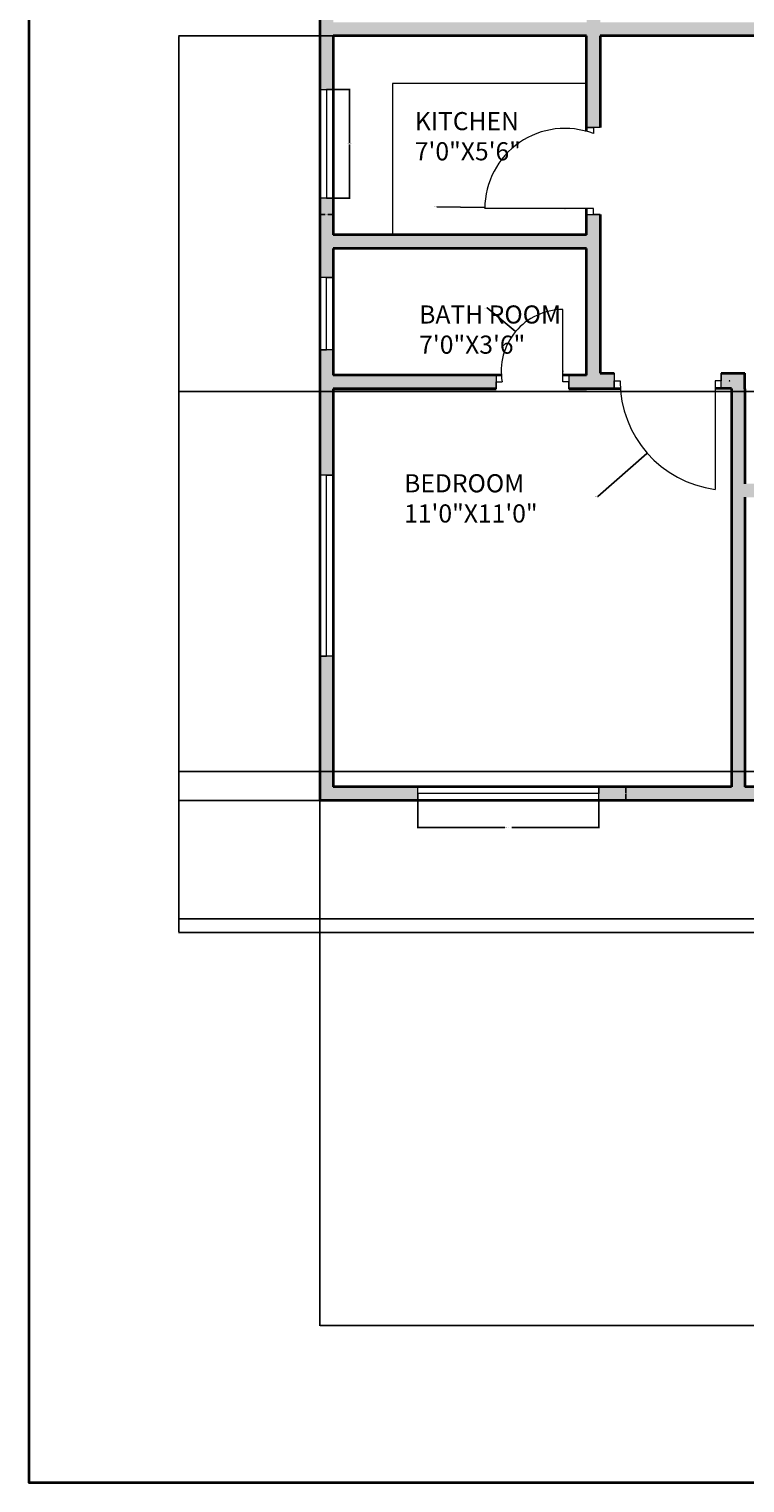
# Model space of a CAD drawing. Units: inches. Extents: x 2314 to 3223, y 1382 to 2735.
# Tile 1 of 14: x 2314 to 2551, y 1382 to 1864. Entities that reach past the tile are written whole.
import ezdxf

# ---------------------------------------------------------------- set-up
doc = ezdxf.new("R2010")
doc.units = ezdxf.units.IN
for name, color, linetype, lineweight in [('A-ANNO-DIMS', 2, 'Continuous', 18), ('A-ANNO-TTLB', 7, 'Continuous', 35), ('A-AREA-IDEN', 7, 'Continuous', 18), ('A-DOOR', 3, 'Continuous', 18), ('A-FLOR-FIXT', 8, 'Continuous', 18), ('A-GLAZ', 4, 'Continuous', 18), ('A-WALL', 7, 'Continuous', 35)]:
    doc.layers.add(name, color=color, linetype=linetype, lineweight=lineweight)
doc.layers.add('A-WALL-PATT', color=251, linetype='Continuous', lineweight=13, true_color=0x636466)
doc.styles.get("Standard").update_dxf_attribs({"font": 'arial.ttf'})
doc.dimstyles.get("Standard").update_dxf_attribs({"dimtxt": 0.18, "dimasz": 0.18, "dimexe": 0.18, "dimexo": 0.0625, "dimgap": 0.09, "dimtad": 0, "dimtih": 1, "dimtoh": 1, "dimdec": 4, "dimzin": 0, "dimdsep": 46, "dimtxsty": 'Standard', "dimcen": 0.09, "dimadec": 0, "dimazin": 0, "dimtfac": 1, "dimtdec": 4, "dimtofl": 0, "dimtmove": 0, "dimatfit": 3, "dimfxl": 1, "dimtolj": 1, "dimtzin": 0, "dimarcsym": 0})

# ---------------------------------------------------------------- blocks, each defined once
blk = doc.blocks.new('WIN-PLAN-24')
for p, q in [((0, 24), (4.5, 24)), ((4.5, 24), (2.25, 24)), ((2.25, 24), (2.25, 0)), ((2.25, 0), (0, 0)), ((0, 0), (4.5, 0))]:
    blk.add_line(p, q)
blk = doc.blocks.new('WIN-PLAN-60')
for p, q in [((0, 4.5), (0, 0)), ((0, 0), (0, 2.25)), ((0, 2.25), (60, 2.25)), ((60, 2.25), (60, 4.5)), ((60, 4.5), (60, 0))]:
    blk.add_line(p, q)
blk = doc.blocks.new('WIN-PLAN-36-ALT')
for p, q in [((0, 36), (4.5, 36)), ((4.5, 36), (2.25, 36)), ((2.25, 36), (2.25, 0)), ((4.5, 0), (0, 0)), ((2.25, 0), (4.5, 0))]:
    blk.add_line(p, q)
blk = doc.blocks.new('*D11')
at = {"layer": 'A-ANNO-DIMS', "color": 0, "lineweight": -2, "transparency": 16777216}
for p, q in [((2442.93, 1608.32), (2442.93, 1599.2)), ((2502.93, 1608.32), (2502.93, 1599.2)), ((2443.11, 1599.38), (2471.82, 1599.38)), ((2502.75, 1599.38), (2474.05, 1599.38))]:
    blk.add_line(p, q, dxfattribs=at)
at = {"layer": 'A-ANNO-DIMS', "color": 0, "transparency": 16777216}
for points in [[(2443.11, 1599.41), (2443.11, 1599.35), (2442.93, 1599.38)], [(2502.75, 1599.41), (2502.75, 1599.35), (2502.93, 1599.38)]]:
    blk.add_solid(points, dxfattribs=at)
at = {"layer": 'Defpoints', "color": 0, "transparency": 16777216}
for p in [(2442.93, 1608.38), (2502.93, 1608.38), (2442.93, 1599.38)]:
    blk.add_point(p, dxfattribs=at)
at = {"layer": 'A-ANNO-DIMS', "color": 0, "transparency": 16777216, "insert": (2472.93, 1599.38), "char_height": 0.18, "attachment_point": 5}
blk.add_mtext('\\A1;WINDOW 60 TYP.', dxfattribs=at)
blk = doc.blocks.new('*D12')
at = {"layer": 'A-ANNO-DIMS', "color": 0, "lineweight": -2, "transparency": 16777216}
for p, q in [((2503, 1612.88), (2512.11, 1612.88)), ((2511.93, 1612.7), (2511.93, 1610.81)), ((2511.93, 1608.56), (2511.93, 1610.45)), ((2503, 1608.38), (2512.11, 1608.38))]:
    blk.add_line(p, q, dxfattribs=at)
at = {"layer": 'A-ANNO-DIMS', "color": 0, "transparency": 16777216}
for points in [[(2511.9, 1612.7), (2511.96, 1612.7), (2511.93, 1612.88)], [(2511.9, 1608.56), (2511.96, 1608.56), (2511.93, 1608.38)]]:
    blk.add_solid(points, dxfattribs=at)
at = {"layer": 'Defpoints', "color": 0, "transparency": 16777216}
for p in [(2502.93, 1612.88), (2502.93, 1608.38), (2511.93, 1608.38)]:
    blk.add_point(p, dxfattribs=at)
at = {"layer": 'A-ANNO-DIMS', "color": 0, "transparency": 16777216, "insert": (2511.93, 1610.63), "char_height": 0.18, "attachment_point": 5}
blk.add_mtext('\\A1;5 TYP.', dxfattribs=at)
blk = doc.blocks.new('*D19')
at = {"layer": 'A-ANNO-DIMS', "color": 0, "lineweight": -2, "transparency": 16777216}
for p, q in [((2414.96, 1844.09), (2420.47, 1844.09)), ((2420.29, 1843.91), (2420.29, 1826.28)), ((2420.29, 1808.27), (2420.29, 1825.91)), ((2414.96, 1808.09), (2420.47, 1808.09))]:
    blk.add_line(p, q, dxfattribs=at)
at = {"layer": 'A-ANNO-DIMS', "color": 0, "transparency": 16777216}
for points in [[(2420.26, 1843.91), (2420.32, 1843.91), (2420.29, 1844.09)], [(2420.26, 1808.27), (2420.32, 1808.27), (2420.29, 1808.09)]]:
    blk.add_solid(points, dxfattribs=at)
at = {"layer": 'Defpoints', "color": 0, "transparency": 16777216}
for p in [(2414.89, 1844.09), (2420.29, 1844.09), (2414.89, 1808.09)]:
    blk.add_point(p, dxfattribs=at)
at = {"layer": 'A-ANNO-DIMS', "color": 0, "transparency": 16777216, "insert": (2420.29, 1826.09), "char_height": 0.18, "attachment_point": 5}
blk.add_mtext('\\A1;WINDOW 36 TYP.', dxfattribs=at)
blk = doc.blocks.new('*D20')
at = {"layer": 'A-ANNO-DIMS', "color": 0, "lineweight": -2, "transparency": 16777216}
for p, q in [((2410.39, 1808.03), (2410.39, 1802.51)), ((2414.89, 1808.03), (2414.89, 1802.51)), ((2410.57, 1802.69), (2412.18, 1802.69)), ((2414.71, 1802.69), (2413.1, 1802.69))]:
    blk.add_line(p, q, dxfattribs=at)
at = {"layer": 'A-ANNO-DIMS', "color": 0, "transparency": 16777216}
for points in [[(2410.57, 1802.72), (2410.57, 1802.66), (2410.39, 1802.69)], [(2414.71, 1802.72), (2414.71, 1802.66), (2414.89, 1802.69)]]:
    blk.add_solid(points, dxfattribs=at)
at = {"layer": 'Defpoints', "color": 0, "transparency": 16777216}
for p in [(2410.39, 1808.09), (2414.89, 1808.09), (2414.89, 1802.69)]:
    blk.add_point(p, dxfattribs=at)
at = {"layer": 'A-ANNO-DIMS', "color": 0, "transparency": 16777216, "insert": (2412.64, 1802.69), "char_height": 0.18, "attachment_point": 5}
blk.add_mtext('\\A1;5 TYP.', dxfattribs=at)
blk = doc.blocks.new('*D29')
at = {"layer": 'A-ANNO-DIMS', "color": 0, "lineweight": -2, "transparency": 16777216}
for p, q in [((2410.39, 1608.32), (2410.39, 1434.13)), ((3125.89, 1608.32), (3125.89, 1434.13)), ((2410.57, 1434.31), (2767.75, 1434.31)), ((3125.71, 1434.31), (2768.54, 1434.31))]:
    blk.add_line(p, q, dxfattribs=at)
at = {"layer": 'A-ANNO-DIMS', "color": 0, "transparency": 16777216}
for points in [[(2410.57, 1434.34), (2410.57, 1434.28), (2410.39, 1434.31)], [(3125.71, 1434.34), (3125.71, 1434.28), (3125.89, 1434.31)]]:
    blk.add_solid(points, dxfattribs=at)
at = {"layer": 'Defpoints', "color": 0, "transparency": 16777216}
for p in [(2410.39, 1608.38), (3125.89, 1608.38), (3125.89, 1434.31)]:
    blk.add_point(p, dxfattribs=at)
at = {"layer": 'A-ANNO-DIMS', "color": 0, "transparency": 16777216, "insert": (2768.14, 1434.31), "char_height": 0.18, "attachment_point": 5}
blk.add_mtext('\\A1;715.5', dxfattribs=at)
blk = doc.blocks.new('*D31')
at = {"layer": 'A-ANNO-DIMS', "color": 0, "lineweight": -2, "transparency": 16777216}
for p, q in [((2410.33, 1608.38), (2363.51, 1608.38)), ((2363.69, 1608.2), (2363.69, 1586.68)), ((2363.69, 1564.8), (2363.69, 1586.32)), ((2717.83, 1564.62), (2363.51, 1564.62))]:
    blk.add_line(p, q, dxfattribs=at)
at = {"layer": 'A-ANNO-DIMS', "color": 0, "transparency": 16777216}
for points in [[(2363.66, 1608.2), (2363.72, 1608.2), (2363.69, 1608.38)], [(2363.66, 1564.8), (2363.72, 1564.8), (2363.69, 1564.62)]]:
    blk.add_solid(points, dxfattribs=at)
at = {"layer": 'Defpoints', "color": 0, "transparency": 16777216}
for p in [(2363.69, 1608.38), (2410.39, 1608.38), (2717.89, 1564.62)]:
    blk.add_point(p, dxfattribs=at)
at = {"layer": 'A-ANNO-DIMS', "color": 0, "transparency": 16777216, "insert": (2363.69, 1586.5), "char_height": 0.18, "attachment_point": 5}
blk.add_mtext('\\A1;43.76', dxfattribs=at)
blk = doc.blocks.new('*D32')
at = {"layer": 'A-ANNO-DIMS', "color": 0, "lineweight": -2, "transparency": 16777216}
for p, q in [((2414.83, 1861.88), (2363.51, 1861.88)), ((2363.69, 1861.7), (2363.69, 1735.32)), ((2363.69, 1608.56), (2363.69, 1734.95)), ((2410.33, 1608.38), (2363.51, 1608.38))]:
    blk.add_line(p, q, dxfattribs=at)
at = {"layer": 'A-ANNO-DIMS', "color": 0, "transparency": 16777216}
for points in [[(2363.66, 1861.7), (2363.72, 1861.7), (2363.69, 1861.88)], [(2363.66, 1608.56), (2363.72, 1608.56), (2363.69, 1608.38)]]:
    blk.add_solid(points, dxfattribs=at)
at = {"layer": 'Defpoints', "color": 0, "transparency": 16777216}
for p in [(2363.69, 1861.88), (2414.89, 1861.88), (2410.39, 1608.38)]:
    blk.add_point(p, dxfattribs=at)
at = {"layer": 'A-ANNO-DIMS', "color": 0, "transparency": 16777216, "insert": (2363.69, 1735.13), "char_height": 0.18, "attachment_point": 5}
blk.add_mtext('\\A1;253.5', dxfattribs=at)
blk = doc.blocks.new('*D35')
at = {"layer": 'A-ANNO-DIMS', "color": 0, "lineweight": -2, "transparency": 16777216}
for p, q in [((2722.33, 1744), (2363.51, 1744)), ((2363.69, 1743.82), (2363.69, 1681.18)), ((2363.69, 1618.18), (2363.69, 1680.82)), ((2722.33, 1618), (2363.51, 1618))]:
    blk.add_line(p, q, dxfattribs=at)
at = {"layer": 'A-ANNO-DIMS', "color": 0, "transparency": 16777216}
for points in [[(2363.66, 1743.82), (2363.72, 1743.82), (2363.69, 1744)], [(2363.66, 1618.18), (2363.72, 1618.18), (2363.69, 1618)]]:
    blk.add_solid(points, dxfattribs=at)
at = {"layer": 'Defpoints', "color": 0, "transparency": 16777216}
for p in [(2363.69, 1744), (2722.39, 1744), (2722.39, 1618)]:
    blk.add_point(p, dxfattribs=at)
at = {"layer": 'A-ANNO-DIMS', "color": 0, "transparency": 16777216, "insert": (2363.69, 1681), "char_height": 0.18, "attachment_point": 5}
blk.add_mtext('\\A1;126', dxfattribs=at)
blk = doc.blocks.new('*D36')
at = {"layer": 'A-ANNO-DIMS', "color": 0, "lineweight": -2, "transparency": 16777216}
for p, q in [((2722.33, 1618), (2363.51, 1618)), ((2363.69, 1617.82), (2363.69, 1593.74)), ((2363.69, 1569.3), (2363.69, 1593.38)), ((2722.33, 1569.12), (2363.51, 1569.12))]:
    blk.add_line(p, q, dxfattribs=at)
at = {"layer": 'A-ANNO-DIMS', "color": 0, "transparency": 16777216}
for points in [[(2363.66, 1617.82), (2363.72, 1617.82), (2363.69, 1618)], [(2363.66, 1569.3), (2363.72, 1569.3), (2363.69, 1569.12)]]:
    blk.add_solid(points, dxfattribs=at)
at = {"layer": 'Defpoints', "color": 0, "transparency": 16777216}
for p in [(2363.69, 1618), (2722.39, 1618), (2722.39, 1569.12)]:
    blk.add_point(p, dxfattribs=at)
at = {"layer": 'A-ANNO-DIMS', "color": 0, "transparency": 16777216, "insert": (2363.69, 1593.56), "char_height": 0.18, "attachment_point": 5}
blk.add_mtext('\\A1;48.88', dxfattribs=at)
blk = doc.blocks.new('*D63')
at = {"layer": 'A-ANNO-DIMS', "color": 0, "lineweight": -2, "transparency": 16777216}
for p, q in [((2546.17, 1747.46), (2546.35, 1747.46)), ((2546.26, 1747.37), (2546.26, 1747.55)), ((2502.67, 1709.19), (2518.88, 1723.42)), ((2502.49, 1709.19), (2502.67, 1709.19))]:
    blk.add_line(p, q, dxfattribs=at)
at = {"layer": 'A-ANNO-DIMS', "color": 0, "transparency": 16777216}
blk.add_solid([(2518.86, 1723.44), (2518.9, 1723.4), (2519.02, 1723.54)], dxfattribs=at)
at = {"layer": 'Defpoints', "color": 0, "transparency": 16777216}
for p in [(2546.26, 1747.46), (2519.02, 1723.54)]:
    blk.add_point(p, dxfattribs=at)
at = {"layer": 'A-ANNO-DIMS', "color": 0, "transparency": 16777216, "insert": (2502.01, 1709.19), "char_height": 0.18, "attachment_point": 5}
blk.add_mtext('\\A1;R36.25', dxfattribs=at)
blk = doc.blocks.new('*D77')
at = {"layer": 'A-ANNO-DIMS', "color": 0, "lineweight": -2, "transparency": 16777216}
for p, q in [((2449.2, 1805.22), (2464.97, 1805)), ((2491.62, 1804.64), (2491.8, 1804.64)), ((2491.71, 1804.55), (2491.71, 1804.73))]:
    blk.add_line(p, q, dxfattribs=at)
at = {"layer": 'A-ANNO-DIMS', "color": 0, "transparency": 16777216}
blk.add_solid([(2464.97, 1805.03), (2464.96, 1804.97), (2465.15, 1805)], dxfattribs=at)
at = {"layer": 'Defpoints', "color": 0, "transparency": 16777216}
for p in [(2465.15, 1805), (2491.71, 1804.64)]:
    blk.add_point(p, dxfattribs=at)
at = {"layer": 'A-ANNO-DIMS', "color": 0, "transparency": 16777216, "insert": (2448.72, 1805.22), "char_height": 0.18, "attachment_point": 5}
blk.add_mtext('\\A1;R26.57', dxfattribs=at)
blk = doc.blocks.new('*D87')
at = {"layer": 'A-ANNO-DIMS', "color": 0, "lineweight": -2, "transparency": 16777216}
for p, q in [((2465.76, 1771.68), (2465.94, 1771.68)), ((2465.94, 1771.68), (2475.19, 1763.94)), ((2490.89, 1750.73), (2491.07, 1750.73)), ((2490.98, 1750.64), (2490.98, 1750.82))]:
    blk.add_line(p, q, dxfattribs=at)
at = {"layer": 'A-ANNO-DIMS', "color": 0, "transparency": 16777216}
blk.add_solid([(2475.21, 1763.96), (2475.17, 1763.92), (2475.33, 1763.82)], dxfattribs=at)
at = {"layer": 'Defpoints', "color": 0, "transparency": 16777216}
for p in [(2475.33, 1763.82), (2490.98, 1750.73)]:
    blk.add_point(p, dxfattribs=at)
at = {"layer": 'A-ANNO-DIMS', "color": 0, "transparency": 16777216, "insert": (2465.21, 1771.68), "char_height": 0.18, "attachment_point": 5}
blk.add_mtext('\\A1;R20.408', dxfattribs=at)

msp = doc.modelspace()

# ---------------------------------------------------------------- hatches: boundary and pattern name
at = {"layer": 'A-WALL-PATT'}
h = msp.add_hatch(color=256, dxfattribs=at)
h.dxf.hatch_style = 1
h.paths.add_polyline_path([(2443.3302, 2379.5332), (2443.3302, 2381.7832), (2410.3927, 2381.7832), (2410.3927, 2336.7008), (2414.8927, 2336.7008), (2414.8927, 2377.2832), (2443.3302, 2377.2832)])
h.paths.add_polyline_path([(2561.3645, 2379.5332), (2561.3645, 2381.7832), (2503.3302, 2381.7832), (2503.3302, 2377.2832), (2546.8927, 2377.2832), (2546.8927, 2245.2832), (2541.8787, 2245.2832), (2541.8787, 2240.7832), (2551.3927, 2240.7832), (2551.3927, 2377.2832), (2561.3645, 2377.2832)])
h.paths.add_polyline_path([(2656.0607, 2381.7832), (2597.3645, 2381.7832), (2597.3645, 2377.2832), (2617.3927, 2377.2832), (2617.3927, 2257.2832), (2584.2532, 2257.2832), (2584.2532, 2252.7832), (2625.8528, 2252.7832), (2625.8528, 2255.0332), (2625.8528, 2257.2832), (2621.8927, 2257.2832), (2621.8927, 2377.2832), (2656.0607, 2377.2832), (2656.0607, 2379.5332)])
h.paths.add_polyline_path([(2807.3418, 2381.7832), (2716.0607, 2381.7832), (2716.0607, 2377.2832), (2765.8927, 2377.2832), (2765.8927, 2257.2832), (2661.6935, 2257.2832), (2661.6935, 2252.7832), (2765.8927, 2252.7832), (2765.8927, 2146.2832), (2760.9259, 2146.2832), (2760.9259, 2141.8832), (2775.7119, 2141.8832), (2775.7119, 2146.2832), (2770.3927, 2146.2832), (2770.3927, 2252.7832), (2877.684, 2252.7832), (2877.684, 2255.0332), (2877.684, 2257.2832), (2770.3927, 2257.2832), (2770.3927, 2377.2832), (2807.3418, 2377.2832), (2807.3418, 2379.5332)])
h.paths.add_polyline_path([(2937.2118, 2381.7832), (2867.3418, 2381.7832), (2867.3418, 2377.2832), (2914.3927, 2377.2832), (2914.3927, 2257.2832), (2908.4124, 2257.2832), (2908.4124, 2252.7832), (2960.6432, 2252.7832), (2960.6432, 2255.0332), (2960.6432, 2257.2832), (2918.8927, 2257.2832), (2918.8927, 2377.2832), (2937.2118, 2377.2832)])
h.paths.add_polyline_path([(3022.1601, 2381.7832), (2973.2118, 2381.7832), (2973.2118, 2379.5332), (2973.2118, 2377.2832), (2984.8927, 2377.2832), (2984.8927, 2257.2832), (2980.0601, 2257.2832), (2980.0601, 2252.7832), (2984.8927, 2252.7832), (2984.8927, 2240.7832), (2995.668, 2240.7832), (2995.668, 2243.0332), (2995.668, 2245.2832), (2989.3927, 2245.2832), (2989.3927, 2377.2832), (3022.1601, 2377.2832), (3022.1601, 2379.5332)])
h.paths.add_polyline_path([(3125.8927, 2381.7832), (3082.1601, 2381.7832), (3082.1601, 2377.2832), (3121.3927, 2377.2832), (3121.3927, 2334.7388), (3125.8927, 2334.7388)])
h.paths.add_polyline_path([(3125.8927, 2274.7388), (3121.3927, 2274.7388), (3121.3927, 2245.2832), (3066.4832, 2245.2832), (3066.4832, 2240.7832), (3121.3927, 2240.7832), (3121.3927, 2232.1868), (3125.8927, 2232.1868)])
h.paths.add_polyline_path([(3125.8927, 2208.1868), (3121.3927, 2208.1868), (3121.3927, 2198.7832), (3037.3927, 2198.7832), (3037.3927, 2240.7832), (3041.2694, 2240.7832), (3041.2694, 2243.0332), (3041.2694, 2245.2832), (3026.8205, 2245.2832), (3026.8205, 2240.7832), (3032.8927, 2240.7832), (3032.8927, 2190.4022), (3037.3927, 2190.4022), (3037.3927, 2194.2832), (3121.3927, 2194.2832), (3121.3927, 2182.1835), (3125.8927, 2182.1835)])
h.paths.add_polyline_path([(3125.8927, 2158.1835), (3121.3927, 2158.1835), (3121.3927, 2146.2832), (3037.3927, 2146.2832), (3037.3927, 2169.3726), (3035.1427, 2169.3726), (3032.8927, 2169.3726), (3032.8927, 2146.2832), (2812.7301, 2146.2832), (2812.7301, 2144.0832), (2812.7301, 2141.8832), (2818.3927, 2141.8832), (2818.3927, 1970.1316), (2822.8927, 1970.1316), (2822.8927, 1978.8832), (2903.9846, 1978.8832), (2903.9846, 1981.1332), (2903.9846, 1983.3832), (2822.8927, 1983.3832), (2822.8927, 2115.3832), (2851.7162, 2115.3832), (2851.7162, 2117.6332), (2851.7162, 2119.8832), (2822.8927, 2119.8832), (2822.8927, 2141.8832), (3125.8927, 2141.8832)])
h.paths.add_polyline_path([(3125.8927, 2119.8832), (3081.193, 2119.8832), (3081.193, 2115.3832), (3121.3927, 2115.3832), (3121.3927, 2071.8188), (3125.8927, 2071.8188)], flags=17)
h.paths.add_polyline_path([(2989.3927, 2115.3832), (3021.193, 2115.3832), (3021.193, 2117.6332), (3021.193, 2119.8832), (2979.123, 2119.8832), (2979.123, 2115.3832), (2984.8927, 2115.3832), (2984.8927, 2019.3832), (2981.9225, 2019.3832), (2981.9225, 2014.8832), (2984.8927, 2014.8832), (2984.8927, 1983.3832), (2984.8927, 1978.8832), (2989.3927, 1978.8832), (2989.3927, 1983.3832)], flags=17)
h.paths.add_polyline_path([(2947.3927, 2115.3832), (2955.123, 2115.3832), (2955.123, 2117.6332), (2955.123, 2119.8832), (2911.7162, 2119.8832), (2911.7162, 2115.3832), (2942.8927, 2115.3832), (2942.8927, 1983.3832), (2936.7017, 1983.3832), (2936.7017, 1978.8832), (2947.3927, 1978.8832), (2947.3927, 1983.3832), (2947.3927, 2014.8832), (2960.7167, 2014.8832), (2960.7167, 2017.1332), (2960.7167, 2019.3832), (2947.3927, 2019.3832)], flags=17)
h.paths.add_polyline_path([(3037.3927, 1978.8832), (3041.8276, 1978.8832), (3041.8276, 1981.1332), (3041.8276, 1983.3832), (3025.477, 1983.3832), (3025.477, 1978.8832), (3032.8927, 1978.8832), (3032.8927, 1927.1259), (3035.1427, 1927.1259), (3037.3927, 1927.1259)])
h.paths.add_polyline_path([(3125.8927, 2011.8188), (3123.6427, 2011.8188), (3121.3927, 2011.8188), (3121.3927, 1983.3832), (3065, 1983.3832), (3065, 1978.8832), (3121.3927, 1978.8832), (3121.3927, 1970.5932), (3125.8927, 1970.5932)], flags=17)
h.paths.add_polyline_path([(2994.2341, 1983.3832), (2989.3927, 1983.3832), (2989.3927, 1978.8832), (2994.2341, 1978.8832), (2994.2341, 1981.1332)], flags=16)
h.paths.add_polyline_path([(3125.8927, 1946.5932), (3121.3927, 1946.5932), (3121.3927, 1936.8832), (3037.3927, 1936.8832), (3037.3927, 1932.3832), (3121.3927, 1932.3832), (3121.3927, 1919.825), (3125.8927, 1919.825)])
h.paths.add_polyline_path([(3125.8927, 1883.825), (3121.3927, 1883.825), (3121.3927, 1866.3832), (3037.3927, 1866.3832), (3037.3927, 1899.0954), (3035.1427, 1899.0954), (3032.8927, 1899.0954), (3032.8927, 1866.3832), (2822.8927, 1866.3832), (2822.8927, 1938.7212), (2820.6427, 1938.7212), (2818.3927, 1938.7212), (2818.3927, 1786.9239), (2822.8927, 1786.9239), (2822.8927, 1861.8832), (3032.8927, 1861.8832), (3032.8927, 1825.1023), (3037.3927, 1825.1023), (3037.3927, 1861.8832), (3121.3927, 1861.8832), (3121.3927, 1844.6765), (3125.8927, 1844.6765)])
h.paths.add_polyline_path([(3125.8927, 1808.6765), (3121.3927, 1808.6765), (3121.3927, 1795.8832), (3037.3927, 1795.8832), (3037.3927, 1799.4755), (3032.8927, 1799.4755), (3032.8927, 1749.3832), (3026.5034, 1749.3832), (3026.5034, 1744.8832), (3032.8927, 1744.8832), (3034.9255, 1744.8832), (3043.1326, 1744.8832), (3043.1326, 1747.1332), (3043.1326, 1749.3832), (3037.3927, 1749.3832), (3037.3927, 1791.3832), (3121.3927, 1791.3832), (3121.3927, 1783.3103), (3125.8927, 1783.3103)])
h.paths.add_polyline_path([(3125.8927, 1759.3103), (3121.3927, 1759.3103), (3121.3927, 1749.3832), (3065.1845, 1749.3832), (3065.1845, 1744.8832), (3121.3927, 1744.8832), (3121.3927, 1709.3573), (3125.8927, 1709.3573)])
h.paths.add_polyline_path([(3125.8927, 1649.3573), (3121.3927, 1649.3573), (3121.3927, 1612.8832), (3095.116, 1612.8832), (3095.116, 1608.3832), (3125.8927, 1608.3832)])
h.paths.add_polyline_path([(3035.116, 1612.8832), (2993.8927, 1612.8832), (2993.8927, 1744.8832), (2998.7409, 1744.8832), (2998.7409, 1749.3832), (2989.3927, 1749.3832), (2989.3927, 1744.8832), (2989.3927, 1701.3832), (2972.8226, 1701.3832), (2972.8226, 1696.8832), (2989.3927, 1696.8832), (2989.3927, 1612.8832), (2978.2225, 1612.8832), (2978.2225, 1608.3832), (3035.116, 1608.3832), (3035.116, 1610.6332)])
h.paths.add_polyline_path([(2947.3927, 1696.8832), (2950.7566, 1696.8832), (2950.7566, 1699.1332), (2950.7566, 1701.3832), (2947.3927, 1701.3832), (2947.3927, 1744.8832), (2947.3927, 1749.3832), (2937.649, 1749.3832), (2937.649, 1744.8832), (2942.8927, 1744.8832), (2942.8927, 1612.8832), (2907.783, 1612.8832), (2907.783, 1608.3832), (2954.2225, 1608.3832), (2954.2225, 1610.6332), (2954.2225, 1612.8832), (2947.3927, 1612.8832)])
h.paths.add_polyline_path([(2822.8927, 1744.8832), (2905.3491, 1744.8832), (2905.3491, 1747.1332), (2905.3491, 1749.3832), (2822.8927, 1749.3832), (2822.8927, 1756.9185), (2818.3927, 1756.9185), (2818.3927, 1612.8832), (2818.3927, 1569.1205), (2722.3927, 1569.1205), (2722.3927, 1612.8832), (2722.3927, 1756.9185), (2717.8927, 1756.9185), (2717.8927, 1750.0143), (2633.6297, 1750.0143), (2633.6437, 1745.2665), (2717.8927, 1745.5143), (2717.8927, 1612.8832), (2689.8467, 1612.8832), (2689.8467, 1608.3832), (2717.8927, 1608.3832), (2717.8927, 1564.6205), (2722.3927, 1564.6205), (2822.8927, 1564.6205), (2822.8927, 1569.1205), (2822.8927, 1608.3832), (2847.783, 1608.3832), (2847.783, 1610.6332), (2847.783, 1612.8832), (2822.8927, 1612.8832)])
h.paths.add_polyline_path([(2629.8467, 1612.8832), (2597.8927, 1612.8832), (2597.8927, 1744.8832), (2597.8927, 1745.1613), (2601.5887, 1745.1721), (2601.5816, 1747.5932), (2601.5745, 1750.0143), (2593.3927, 1750.0143), (2593.3927, 1744.8832), (2593.3927, 1713.3832), (2589.7588, 1713.3832), (2589.7588, 1708.8832), (2593.3927, 1708.8832), (2593.3927, 1612.8832), (2582.3793, 1612.8832), (2582.3793, 1608.3832), (2629.8467, 1608.3832), (2629.8467, 1610.6332)])
h.paths.add_polyline_path([(2551.3927, 1708.8832), (2567.6776, 1708.8832), (2567.6776, 1711.1332), (2567.6776, 1713.3832), (2551.3927, 1713.3832), (2551.3927, 1744.8832), (2551.3927, 1750.0143), (2543.5657, 1750.0143), (2543.5657, 1747.5079), (2543.5657, 1745.0014), (2546.8927, 1745.0112), (2546.8927, 1744.8832), (2546.8927, 1612.8832), (2502.9339, 1612.8832), (2502.9339, 1608.3832), (2558.3793, 1608.3832), (2558.3793, 1610.6332), (2558.3793, 1612.8832), (2551.3927, 1612.8832)])
h.paths.add_polyline_path([(2414.8927, 1656.2547), (2410.3927, 1656.2547), (2410.3927, 1608.3832), (2442.9339, 1608.3832), (2442.9339, 1610.6332), (2442.9339, 1612.8832), (2414.8927, 1612.8832)])
h.paths.add_polyline_path([(2414.8927, 1744.8832), (2468.8906, 1744.8832), (2468.8906, 1747.1332), (2468.8906, 1749.3832), (2414.8927, 1749.3832), (2414.8927, 1757.7622), (2410.3927, 1757.7622), (2410.3927, 1716.2547), (2414.8927, 1716.2547)])
h.paths.add_polyline_path([(2414.8927, 1791.3832), (2498.8927, 1791.3832), (2498.8927, 1749.3832), (2492.9799, 1749.3832), (2492.9799, 1744.8832), (2498.8927, 1744.8832), (2503.3927, 1744.8832), (2508.0135, 1744.8968), (2508.0059, 1747.4556), (2507.9984, 1750.0143), (2503.3927, 1750.0143), (2503.3927, 1802.6362), (2501.1427, 1802.6362), (2498.8927, 1802.6362), (2498.8927, 1795.8832), (2414.8927, 1795.8832), (2414.8927, 1808.0943), (2410.3927, 1808.0943), (2410.3927, 1781.7622), (2414.8927, 1781.7622)])
h.paths.add_polyline_path([(2722.3927, 1937.589), (2720.1427, 1937.589), (2717.8927, 1937.589), (2717.8927, 1866.3832), (2503.3927, 1866.3832), (2503.3927, 1896.3484), (2498.8927, 1896.3484), (2498.8927, 1866.3832), (2414.8927, 1866.3832), (2414.8927, 1882.1496), (2410.3927, 1882.1496), (2410.3927, 1844.0943), (2414.8927, 1844.0943), (2414.8927, 1861.8832), (2498.8927, 1861.8832), (2498.8927, 1831.4783), (2501.1427, 1831.4783), (2503.3927, 1831.4783), (2503.3927, 1861.8832), (2717.8927, 1861.8832), (2717.8927, 1786.9239), (2722.3927, 1786.9239)])
h.paths.add_polyline_path([(2414.8927, 1932.3832), (2498.8927, 1932.3832), (2498.8927, 1924.7883), (2503.3927, 1924.7883), (2503.3927, 1978.8832), (2505.8599, 1978.8832), (2505.8599, 1981.1332), (2505.8599, 1983.3832), (2493.3697, 1983.3832), (2493.3697, 1978.8832), (2498.8927, 1978.8832), (2498.8927, 1936.8832), (2414.8927, 1936.8832), (2414.8927, 1943.2834), (2410.3927, 1943.2834), (2410.3927, 1918.1496), (2414.8927, 1918.1496)])
h.paths.add_polyline_path([(2414.8927, 2020.3133), (2412.6427, 2020.3133), (2410.3927, 2020.3133), (2410.3927, 1967.2834), (2414.8927, 1967.2834), (2414.8927, 1978.8832), (2468.8513, 1978.8832), (2468.8513, 1981.1332), (2468.8513, 1983.3832), (2414.8927, 1983.3832)])
h.paths.add_polyline_path([(2414.8927, 2115.3832), (2453.004, 2115.3832), (2453.004, 2117.6332), (2453.004, 2119.8832), (2410.3927, 2119.8832), (2410.3927, 2080.3133), (2414.8927, 2080.3133)], flags=17)
h.paths.add_polyline_path([(2559.0969, 2117.6332), (2559.0969, 2119.8832), (2513.004, 2119.8832), (2513.004, 2115.3832), (2546.8927, 2115.3832), (2546.8927, 1983.3832), (2542.7531, 1983.3832), (2542.7531, 1978.8832), (2551.3927, 1978.8832), (2551.3927, 2014.8832), (2570.3098, 2014.8832), (2570.3098, 2017.1332), (2570.3098, 2019.3832), (2551.3927, 2019.3832), (2551.3927, 2115.3832), (2559.0969, 2115.3832)], flags=17)
h.paths.add_polyline_path([(2628.5073, 2117.6332), (2628.5073, 2119.8832), (2583.0969, 2119.8832), (2583.0969, 2115.3832), (2593.3927, 2115.3832), (2593.3927, 2019.3832), (2590.2108, 2019.3832), (2590.2108, 2014.8832), (2593.3927, 2014.8832), (2593.3927, 1978.8832), (2601.5907, 1978.8832), (2601.5907, 1981.1332), (2601.5907, 1983.3832), (2597.8927, 1983.3832), (2597.8927, 2115.3832), (2628.5073, 2115.3832)], flags=17)
h.paths.add_polyline_path([(2722.3927, 2141.8832), (2726.9871, 2141.8832), (2726.9871, 2144.2705), (2726.9871, 2146.2832), (2503.3927, 2146.2832), (2503.3927, 2168.2161), (2501.1427, 2168.2161), (2498.8927, 2168.2161), (2498.8927, 2146.2832), (2414.8927, 2146.2832), (2414.8927, 2156.5041), (2410.3927, 2156.5041), (2410.3927, 2141.8832), (2717.8927, 2141.8832), (2717.8927, 2119.8832), (2688.5073, 2119.8832), (2688.5073, 2115.3832), (2717.8927, 2115.3832), (2717.8927, 1983.3832), (2633.2454, 1983.3832), (2633.2454, 1978.8832), (2717.8927, 1978.8832), (2717.8927, 1970.1316), (2720.1427, 1970.1316), (2722.3927, 1970.1316)])
h.paths.add_polyline_path([(2557.3704, 1462.9278), (2940.0934, 1462.9278), (2940.0934, 1512.3848), (2557.3704, 1512.3848)], flags=9)
h.paths.add_polyline_path([(2846.2527, 1703.1384), (2892.8612, 1703.1384), (2892.8612, 1725.5272), (2846.2527, 1725.5272)], flags=25)
h.paths.add_polyline_path([(2885.6102, 1812.1147), (2946.1505, 1812.1147), (2946.1505, 1834.5035), (2885.6102, 1834.5035)], flags=25)
h.paths.add_polyline_path([(2885.6102, 1884.183), (2946.1505, 1884.183), (2946.1505, 1906.5718), (2885.6102, 1906.5718)], flags=25)
h.paths.add_polyline_path([(3066.365, 1705.5431), (3112.9735, 1705.5431), (3112.9735, 1727.9319), (3066.365, 1727.9319)], flags=9)
h.paths.add_polyline_path([(3061.8255, 1887.7513), (3101.6154, 1887.7513), (3101.6154, 1910.1401), (3061.8255, 1910.1401)], flags=25)
h.paths.add_polyline_path([(3063.3679, 1816.2121), (3103.1578, 1816.2121), (3103.1578, 1838.6009), (3063.3679, 1838.6009)], flags=25)
h.paths.add_polyline_path([(3053.3743, 1768.416), (3107.1329, 1768.416), (3107.1329, 1790.8048), (3053.3743, 1790.8048)], flags=25)
h.paths.add_polyline_path([(3061.6068, 1943.822), (3115.3653, 1943.822), (3115.3653, 1966.2109), (3061.6068, 1966.2109)], flags=9)
h.paths.add_polyline_path([(2745.0978, 1763.6604), (2797.9354, 1763.6604), (2797.9354, 1776.0247), (2745.0978, 1776.0247)], flags=9)
h.paths.add_polyline_path([(2574.2135, 1819.2586), (2634.7538, 1819.2586), (2634.7538, 1841.6474), (2574.2135, 1841.6474)], flags=25)
h.paths.add_polyline_path([(2574.2135, 1891.3269), (2634.7538, 1891.3269), (2634.7538, 1913.7157), (2574.2135, 1913.7157)], flags=25)
h.paths.add_polyline_path([(2638.4466, 1702.43), (2685.0551, 1702.43), (2685.0551, 1724.8188), (2638.4466, 1724.8188)], flags=25)
h.paths.add_polyline_path([(2435.9715, 1697.1215), (2482.5799, 1697.1215), (2482.5799, 1719.5103), (2435.9715, 1719.5103)], flags=9)
h.paths.add_polyline_path([(2431.2046, 1893.7833), (2470.9945, 1893.7833), (2470.9945, 1916.1721), (2431.2046, 1916.1721)], flags=25)
h.paths.add_polyline_path([(2439.8144, 1817.2116), (2479.6043, 1817.2116), (2479.6043, 1839.6004), (2439.8144, 1839.6004)], flags=25)
h.paths.add_polyline_path([(2441.2607, 1753.0942), (2495.0192, 1753.0942), (2495.0192, 1775.483), (2441.2607, 1775.483)], flags=25)
h.paths.add_polyline_path([(2421.216, 1945.3109), (2474.9746, 1945.3109), (2474.9746, 1967.6997), (2421.216, 1967.6997)], flags=25)
h.paths.add_polyline_path([(2585.4464, 1627.5703), (2585.4464, 1679), (2563.0576, 1679), (2563.0576, 1627.5703)], flags=9)
h.paths.add_polyline_path([(2978.3497, 1618.7039), (2978.3497, 1670.1337), (2955.9609, 1670.1337), (2955.9609, 1618.7039)], flags=9)
h.paths.add_polyline_path([(2975.9502, 2041.7828), (2975.9502, 2093.2125), (2953.5614, 2093.2125), (2953.5614, 2041.7828)], flags=25)
h.paths.add_polyline_path([(2835.6537, 1989.2068), (2882.2621, 1989.2068), (2882.2621, 2011.5956), (2835.6537, 2011.5956)], flags=25)
h.paths.add_polyline_path([(2649.3769, 1997.5659), (2695.9853, 1997.5659), (2695.9853, 2019.9547), (2649.3769, 2019.9547)], flags=25)
h.paths.add_polyline_path([(2579.9087, 2040.3429), (2579.9087, 2091.7726), (2557.5198, 2091.7726), (2557.5198, 2040.3429)], flags=25)
h.paths.add_polyline_path([(2783.2404, 1883.1956), (2783.2404, 2067.1369), (2764.694, 2067.1369), (2764.694, 1883.1956)], flags=9)
h.paths.add_polyline_path([(3055.8435, 1993.5571), (3102.4519, 1993.5571), (3102.4519, 2015.9459), (3055.8435, 2015.9459)], flags=25)
h.paths.add_polyline_path([(2423.6009, 1984.6082), (2470.2094, 1984.6082), (2470.2094, 2006.997), (2423.6009, 2006.997)], flags=25)
h.paths.add_polyline_path([(2973.4115, 2123.1668), (3013.1319, 2123.1668), (3013.1319, 2135.531), (2973.4115, 2135.531)], flags=25)
h.paths.add_polyline_path([(2534.3846, 2124.6231), (2574.105, 2124.6231), (2574.105, 2136.9874), (2534.3846, 2136.9874)], flags=25)
h.paths.add_polyline_path([(2829.1368, 2188.1931), (2889.411, 2188.1931), (2889.411, 2210.5819), (2829.1368, 2210.5819)], flags=9)
h.paths.add_polyline_path([(2633.2547, 2185.0437), (2693.5289, 2185.0437), (2693.5289, 2207.4325), (2633.2547, 2207.4325)], flags=9)
h.paths.add_polyline_path([(2445.1812, 2167.0395), (2496.611, 2167.0395), (2496.611, 2189.4284), (2445.1812, 2189.4284)], flags=9)
h.paths.add_polyline_path([(2429.1678, 2194.5482), (2480.5975, 2194.5482), (2480.5975, 2216.937), (2429.1678, 2216.937)], flags=9)
h.paths.add_polyline_path([(3060.1138, 2158.1056), (3111.5436, 2158.1056), (3111.5436, 2180.4944), (3060.1138, 2180.4944)], flags=9)
h.paths.add_polyline_path([(3055.6824, 2201.2631), (3107.1122, 2201.2631), (3107.1122, 2223.652), (3055.6824, 2223.652)], flags=25)
h.paths.add_polyline_path([(3044.3482, 2257.7345), (3090.9567, 2257.7345), (3090.9567, 2280.1233), (3044.3482, 2280.1233)], flags=9)
h.paths.add_polyline_path([(2942.5437, 2306.9625), (2982.3336, 2306.9625), (2982.3336, 2329.3513), (2942.5437, 2329.3513)], flags=9)
h.paths.add_polyline_path([(2799.5865, 2259.1663), (2846.195, 2259.1663), (2846.195, 2281.5551), (2799.5865, 2281.5551)], flags=25)
h.paths.add_polyline_path([(2670.4998, 2261.1493), (2717.1082, 2261.1493), (2717.1082, 2283.5381), (2670.4998, 2283.5381)], flags=25)
h.paths.add_polyline_path([(2553.0333, 2302.7735), (2592.8232, 2302.7735), (2592.8232, 2325.1624), (2553.0333, 2325.1624)], flags=9)
h.paths.add_polyline_path([(2432.0288, 2268.6489), (2478.6372, 2268.6489), (2478.6372, 2291.0377), (2432.0288, 2291.0377)], flags=9)
h = msp.add_hatch(color=256, dxfattribs=at)
h.dxf.hatch_style = 1
h.paths.add_polyline_path([(2503.3927, 2240.7832), (2507.7952, 2240.7832), (2507.7952, 2245.2832), (2496.4262, 2245.2832), (2496.4262, 2243.0332), (2496.4262, 2240.7832), (2498.8927, 2240.7832), (2498.8927, 2198.7832), (2414.8927, 2198.7832), (2414.8927, 2206.5718), (2410.3927, 2206.5718), (2410.3927, 2180.5041), (2412.6427, 2180.5041), (2414.8927, 2180.5041), (2414.8927, 2194.2832), (2498.8927, 2194.2832), (2498.8927, 2191.0069), (2503.3927, 2191.0069)])
h.paths.add_polyline_path([(2414.8927, 2276.7008), (2410.3927, 2276.7008), (2410.3927, 2230.5718), (2414.8927, 2230.5718), (2414.8927, 2240.7832), (2474.2564, 2240.7832), (2474.2564, 2243.0332), (2474.2564, 2245.2832), (2414.8927, 2245.2832)])
h.paths.add_polyline_path([(2557.3704, 1462.9278), (2940.0934, 1462.9278), (2940.0934, 1512.3848), (2557.3704, 1512.3848)], flags=9)
h.paths.add_polyline_path([(2846.2527, 1703.1384), (2892.8612, 1703.1384), (2892.8612, 1725.5272), (2846.2527, 1725.5272)], flags=9)
h.paths.add_polyline_path([(2885.6102, 1812.1147), (2946.1505, 1812.1147), (2946.1505, 1834.5035), (2885.6102, 1834.5035)], flags=9)
h.paths.add_polyline_path([(2885.6102, 1884.183), (2946.1505, 1884.183), (2946.1505, 1906.5718), (2885.6102, 1906.5718)], flags=9)
h.paths.add_polyline_path([(3066.365, 1705.5431), (3112.9735, 1705.5431), (3112.9735, 1727.9319), (3066.365, 1727.9319)], flags=9)
h.paths.add_polyline_path([(3061.8255, 1887.7513), (3101.6154, 1887.7513), (3101.6154, 1910.1401), (3061.8255, 1910.1401)], flags=9)
h.paths.add_polyline_path([(3063.3679, 1816.2121), (3103.1578, 1816.2121), (3103.1578, 1838.6009), (3063.3679, 1838.6009)], flags=9)
h.paths.add_polyline_path([(3053.3743, 1768.416), (3107.1329, 1768.416), (3107.1329, 1790.8048), (3053.3743, 1790.8048)], flags=9)
h.paths.add_polyline_path([(3061.6068, 1943.822), (3115.3653, 1943.822), (3115.3653, 1966.2109), (3061.6068, 1966.2109)], flags=9)
h.paths.add_polyline_path([(2745.0978, 1763.6604), (2797.9354, 1763.6604), (2797.9354, 1776.0247), (2745.0978, 1776.0247)], flags=9)
h.paths.add_polyline_path([(2574.2135, 1819.2586), (2634.7538, 1819.2586), (2634.7538, 1841.6474), (2574.2135, 1841.6474)], flags=9)
h.paths.add_polyline_path([(2574.2135, 1891.3269), (2634.7538, 1891.3269), (2634.7538, 1913.7157), (2574.2135, 1913.7157)], flags=9)
h.paths.add_polyline_path([(2638.4466, 1702.43), (2685.0551, 1702.43), (2685.0551, 1724.8188), (2638.4466, 1724.8188)], flags=9)
h.paths.add_polyline_path([(2435.9715, 1697.1215), (2482.5799, 1697.1215), (2482.5799, 1719.5103), (2435.9715, 1719.5103)], flags=9)
h.paths.add_polyline_path([(2431.2046, 1893.7833), (2470.9945, 1893.7833), (2470.9945, 1916.1721), (2431.2046, 1916.1721)], flags=9)
h.paths.add_polyline_path([(2439.8144, 1817.2116), (2479.6043, 1817.2116), (2479.6043, 1839.6004), (2439.8144, 1839.6004)], flags=9)
h.paths.add_polyline_path([(2441.2607, 1753.0942), (2495.0192, 1753.0942), (2495.0192, 1775.483), (2441.2607, 1775.483)], flags=9)
h.paths.add_polyline_path([(2421.216, 1945.3109), (2474.9746, 1945.3109), (2474.9746, 1967.6997), (2421.216, 1967.6997)], flags=9)
h.paths.add_polyline_path([(2585.4464, 1627.5703), (2585.4464, 1679), (2563.0576, 1679), (2563.0576, 1627.5703)], flags=9)
h.paths.add_polyline_path([(2978.3497, 1618.7039), (2978.3497, 1670.1337), (2955.9609, 1670.1337), (2955.9609, 1618.7039)], flags=9)
h.paths.add_polyline_path([(2975.9502, 2041.7828), (2975.9502, 2093.2125), (2953.5614, 2093.2125), (2953.5614, 2041.7828)], flags=9)
h.paths.add_polyline_path([(2835.6537, 1989.2068), (2882.2621, 1989.2068), (2882.2621, 2011.5956), (2835.6537, 2011.5956)], flags=9)
h.paths.add_polyline_path([(2649.3769, 1997.5659), (2695.9853, 1997.5659), (2695.9853, 2019.9547), (2649.3769, 2019.9547)], flags=9)
h.paths.add_polyline_path([(2579.9087, 2040.3429), (2579.9087, 2091.7726), (2557.5198, 2091.7726), (2557.5198, 2040.3429)], flags=9)
h.paths.add_polyline_path([(2783.2404, 1883.1956), (2783.2404, 2067.1369), (2764.694, 2067.1369), (2764.694, 1883.1956)], flags=9)
h.paths.add_polyline_path([(3055.8435, 1993.5571), (3102.4519, 1993.5571), (3102.4519, 2015.9459), (3055.8435, 2015.9459)], flags=9)
h.paths.add_polyline_path([(2423.6009, 1984.6082), (2470.2094, 1984.6082), (2470.2094, 2006.997), (2423.6009, 2006.997)], flags=9)
h.paths.add_polyline_path([(2973.4115, 2123.1668), (3013.1319, 2123.1668), (3013.1319, 2135.531), (2973.4115, 2135.531)], flags=9)
h.paths.add_polyline_path([(2534.3846, 2124.6231), (2574.105, 2124.6231), (2574.105, 2136.9874), (2534.3846, 2136.9874)], flags=9)
h.paths.add_polyline_path([(2829.1368, 2188.1931), (2889.411, 2188.1931), (2889.411, 2210.5819), (2829.1368, 2210.5819)], flags=9)
h.paths.add_polyline_path([(2633.2547, 2185.0437), (2693.5289, 2185.0437), (2693.5289, 2207.4325), (2633.2547, 2207.4325)], flags=9)
h.paths.add_polyline_path([(2445.1812, 2167.0395), (2496.611, 2167.0395), (2496.611, 2189.4284), (2445.1812, 2189.4284)], flags=9)
h.paths.add_polyline_path([(2429.1678, 2208.3022), (2480.5975, 2208.3022), (2480.5975, 2230.691), (2429.1678, 2230.691)], flags=25)
h.paths.add_polyline_path([(3060.1138, 2158.1056), (3111.5436, 2158.1056), (3111.5436, 2180.4944), (3060.1138, 2180.4944)], flags=9)
h.paths.add_polyline_path([(3055.6824, 2201.2631), (3107.1122, 2201.2631), (3107.1122, 2223.652), (3055.6824, 2223.652)], flags=9)
h.paths.add_polyline_path([(3044.3482, 2257.7345), (3090.9567, 2257.7345), (3090.9567, 2280.1233), (3044.3482, 2280.1233)], flags=9)
h.paths.add_polyline_path([(2942.5437, 2306.9625), (2982.3336, 2306.9625), (2982.3336, 2329.3513), (2942.5437, 2329.3513)], flags=9)
h.paths.add_polyline_path([(2799.5865, 2259.1663), (2846.195, 2259.1663), (2846.195, 2281.5551), (2799.5865, 2281.5551)], flags=9)
h.paths.add_polyline_path([(2670.4998, 2261.1493), (2717.1082, 2261.1493), (2717.1082, 2283.5381), (2670.4998, 2283.5381)], flags=9)
h.paths.add_polyline_path([(2553.0333, 2302.7735), (2592.8232, 2302.7735), (2592.8232, 2325.1624), (2553.0333, 2325.1624)], flags=9)
h.paths.add_polyline_path([(2432.0288, 2268.6489), (2478.6372, 2268.6489), (2478.6372, 2291.0377), (2432.0288, 2291.0377)], flags=9)

# ---------------------------------------------------------------- linework, layer by layer
at = {"layer": 'A-ANNO-TTLB'}
msp.add_lwpolyline([(2314.008, 2735.417), (3222.6676, 2735.417), (3222.6676, 1382.0876), (2314.008, 1382.0876)], close=True, dxfattribs=at)
at = {"layer": 'A-DOOR'}
for p, q in [((2503.3927, 1831.4783), (2498.8927, 1831.4783)), ((2498.8927, 1831.4783), (2501.1427, 1831.4783)), ((2501.1427, 1831.4783), (2501.1427, 1829.4783)), ((2501.1427, 1804.6362), (2465.1427, 1804.6362)), ((2501.1427, 1802.6362), (2501.1427, 1804.6362)), ((2498.8927, 1802.6362), (2503.3927, 1802.6362)), ((2503.3927, 1802.6362), (2501.1427, 1802.6362)), ((2490.9799, 1747.1332), (2490.9799, 1771.1332)), ((2507.9984, 1750.0143), (2508.0135, 1744.8968)), ((2543.5657, 1745.0014), (2543.5657, 1750.0143)), ((2543.5657, 1750.0143), (2543.5657, 1747.5079)), ((2468.8906, 1749.3832), (2468.8906, 1744.8832)), ((2468.8906, 1744.8832), (2468.8906, 1747.1332)), ((2468.8906, 1747.1332), (2470.8906, 1747.1332)), ((2492.9799, 1747.1332), (2490.9799, 1747.1332)), ((2492.9799, 1749.3832), (2492.9799, 1744.8832)), ((2492.9799, 1744.8832), (2492.9799, 1747.1332)), ((2508.0135, 1744.8968), (2508.0059, 1747.4556)), ((2508.0059, 1747.4556), (2510.0059, 1747.4556)), ((2543.5657, 1747.5079), (2541.5657, 1747.5079)), ((2541.5657, 1747.5079), (2541.5657, 1711.5079))]:
    msp.add_line(p, q, dxfattribs=at)
for centre, radius, start, end in [((2491.7139, 1804.6362), 26.5713, 69.21595, 180), ((2490.9799, 1750.7253), 20.4079, 90, 190.137607), ((2546.2587, 1747.4556), 36.2527, 180, 262.56207)]:
    msp.add_arc(centre, radius, start, end, dxfattribs=at)
at = {"layer": 'A-FLOR-FIXT'}
for p, q in [((2498.8927, 1846.0513), (2434.5377, 1846.0513)), ((2434.5377, 1846.0513), (2434.5377, 1795.8832))]:
    msp.add_line(p, q, dxfattribs=at)
at = {"layer": 'A-WALL'}
for p, q in [((2410.3927, 2119.8832), (2410.3927, 1608.3832)), ((2498.8927, 1861.8832), (2414.8927, 1861.8832)), ((2414.8927, 1861.8832), (2414.8927, 1795.8832)), ((2498.8927, 1830.2193), (2498.8927, 1861.8832)), ((2717.8927, 1861.8832), (2503.3927, 1861.8832)), ((2503.3927, 1861.8832), (2503.3927, 1831.4783)), ((2498.8927, 1795.8832), (2498.8927, 1804.6362)), ((2503.3927, 1802.6362), (2503.3927, 1750.0143)), ((2498.8927, 1795.8832), (2414.8927, 1795.8832)), ((2498.8927, 1791.3832), (2414.8927, 1791.3832)), ((2414.8927, 1791.3832), (2414.8927, 1749.3832)), ((2498.8927, 1749.3832), (2498.8927, 1791.3832)), ((2503.3927, 1750.0143), (2507.9984, 1750.0143)), ((2543.5657, 1750.0143), (2551.3927, 1750.0143)), ((2551.3927, 1744.8832), (2551.3927, 1750.0143)), ((2470.6161, 1749.3832), (2414.8927, 1749.3832)), ((2498.8927, 1749.3832), (2490.9799, 1749.3832)), ((2546.8927, 1745.0112), (2541.5657, 1744.9955)), ((2546.8927, 1744.8832), (2546.8927, 1745.0112)), ((2414.8927, 1744.8832), (2468.8906, 1744.8832)), ((2414.8927, 1744.8832), (2414.8927, 1612.8832)), ((2468.8906, 1744.8832), (2414.8927, 1744.8832)), ((2503.3927, 1744.8832), (2492.9799, 1744.8832)), ((2492.9799, 1744.8832), (2498.8927, 1744.8832)), ((2510.0959, 1744.903), (2503.3927, 1744.8832)), ((2546.8927, 1744.8832), (2546.8927, 1612.8832)), ((2551.3927, 1744.8832), (2551.3927, 1713.3832)), ((2551.3927, 1708.8832), (2551.3927, 1612.8832)), ((2546.8927, 1612.8832), (2414.8927, 1612.8832)), ((2593.3927, 1612.8832), (2551.3927, 1612.8832)), ((2717.8927, 1608.3832), (2410.3927, 1608.3832))]:
    msp.add_line(p, q, dxfattribs=at)

# ---------------------------------------------------------------- block references
at = {"layer": 'A-GLAZ'}
msp.add_blockref('WIN-PLAN-36-ALT', (2410.3927, 1808.0943), dxfattribs=at)
at = {"layer": 'A-GLAZ', "rotation": 180}
for name, p in [('WIN-PLAN-24', (2414.8927, 1781.7622)), ('WIN-PLAN-60', (2502.9339, 1612.8832))]:
    msp.add_blockref(name, p, dxfattribs=at)
at = {"layer": 'A-GLAZ', "extrusion": (0, 0, -1), "zscale": -1, "rotation": 90}
msp.add_blockref('WIN-PLAN-60', (-2410.3927, 1656.2547), dxfattribs=at)

# ---------------------------------------------------------------- texts
at = {"layer": 'A-AREA-IDEN', "char_height": 6, "attachment_point": 1}
for s, width, insert in [('KITCHEN\\P7\'0"X5\'6"', 72.610778, (2441.9283, 1836.6147)), ('BATH ROOM \\P7\'0"X3\'6"', 123.53461, (2443.3746, 1772.5014)), ('BEDROOM\\P11\'0"X11\'0"', 149.374676, (2438.3841, 1716.5287))]:
    msp.add_mtext_dynamic_manual_height_columns(s, width=width, gutter_width=12.5, heights=[0], dxfattribs=dict(at, insert=insert))

# ---------------------------------------------------------------- dimensions: what is measured, and where the dimension line sits
at = {"layer": 'A-ANNO-DIMS'}
for base, p1, p2, override, picture, middle in [((2363.6927, 1861.8832), (2410.3927, 1608.3832), (2414.8927, 1861.8832), {"dimdec": 1, "dimlfac": 1, "dimrnd": 0, "dimzin": 0, "dimdsep": 46, "dimlunit": 2}, '*D32', (2363.6927, 1735.1332)), ((2363.6927, 1743.998), (2722.3927, 1617.998), (2722.3927, 1743.998), {"dimdec": 0, "dimlfac": 1, "dimrnd": 0, "dimzin": 0, "dimdsep": 46, "dimlunit": 2}, '*D35', (2363.6927, 1680.998)), ((2363.6927, 1617.998), (2722.3927, 1569.1205), (2722.3927, 1617.998), {"dimdec": 2, "dimlfac": 1, "dimrnd": 0, "dimzin": 0, "dimdsep": 46, "dimlunit": 2}, '*D36', (2363.6927, 1593.5592)), ((2363.6927, 1608.3832), (2717.8927, 1564.6205), (2410.3927, 1608.3832), {"dimdec": 2, "dimlfac": 1, "dimrnd": 0, "dimzin": 0, "dimdsep": 46, "dimlunit": 2}, '*D31', (2363.6927, 1586.5019))]:
    dim = msp.add_linear_dim(base=base, p1=p1, p2=p2, angle=90, dimstyle='Standard', override=override, dxfattribs=at)
    dim.commit()
    dim.dimension.update_dxf_attribs({"geometry": picture, "text_midpoint": middle})
for base, p1, p2, angle, text, picture, middle in [((2420.2927, 1844.0943), (2414.8927, 1808.0943), (2414.8927, 1844.0943), 90, 'WINDOW <> TYP.', '*D19', (2420.2927, 1826.0943)), ((2511.9338661467, 1608.3832367368), (2502.9338661467, 1612.8832367368), (2502.9338661467, 1608.3832367368), 270, '<> TYP.', '*D12', (2511.9338661467, 1610.6332367368)), ((2442.9339, 1599.3832), (2502.9339, 1608.3832), (2442.9339, 1608.3832), 180, 'WINDOW <> TYP.', '*D11', (2472.9339, 1599.3832))]:
    dim = msp.add_linear_dim(base=base, p1=p1, p2=p2, angle=angle, text=text, dimstyle='Standard', override={"dimdec": 0, "dimlfac": 1, "dimrnd": 0, "dimzin": 0, "dimdsep": 46, "dimlunit": 2}, dxfattribs=at)
    dim.commit()
    dim.dimension.update_dxf_attribs({"geometry": picture, "text_midpoint": middle})
dim = msp.add_linear_dim(base=(2414.8926767707, 1802.6942739264), p1=(2410.3926767707, 1808.0942739264), p2=(2414.8926767707, 1808.0942739264), text='<> TYP.', dimstyle='Standard', override={"dimdec": 0, "dimlfac": 1, "dimrnd": 0, "dimzin": 0, "dimdsep": 46, "dimlunit": 2}, dxfattribs=at)
dim.commit()
dim.dimension.update_dxf_attribs({"geometry": '*D20', "text_midpoint": (2412.6426767707, 1802.6942739264)})
for center, mpoint, override, picture, middle in [((2491.7139, 1804.6362), (2465.1451, 1804.998), {"dimdec": 2, "dimlfac": 1, "dimrnd": 0, "dimzin": 0, "dimdsep": 46, "dimlunit": 2}, '*D77', (2449.2039, 1805.2151)), ((2490.9799, 1750.7253), (2475.3306, 1763.8243), {"dimdec": 3, "dimlfac": 1, "dimrnd": 0, "dimzin": 0, "dimdsep": 46, "dimlunit": 2}, '*D87', (2465.2111, 1771.6837)), ((2546.2587, 1747.4556), (2519.0151, 1723.5381), {"dimdec": 2, "dimlfac": 1, "dimrnd": 0, "dimzin": 0, "dimdsep": 46, "dimlunit": 2}, '*D63', (2502.0084, 1709.1876))]:
    dim = msp.add_radius_dim(center=center, mpoint=mpoint, dimstyle='Standard', override=override, dxfattribs=at)
    dim.commit()
    dim.dimension.update_dxf_attribs({"geometry": picture, "text_midpoint": middle, "dimtype": 164})
dim = msp.add_linear_dim(base=(3125.8927, 1434.3145), p1=(2410.3927, 1608.3832), p2=(3125.8927, 1608.3832), dimstyle='Standard', override={"dimdec": 1, "dimlfac": 1, "dimrnd": 0, "dimzin": 0, "dimdsep": 46, "dimlunit": 2}, dxfattribs=at)
dim.commit()
dim.dimension.update_dxf_attribs({"geometry": '*D29', "text_midpoint": (2768.1427, 1434.3145)})

doc.saveas('drawing.dxf')
